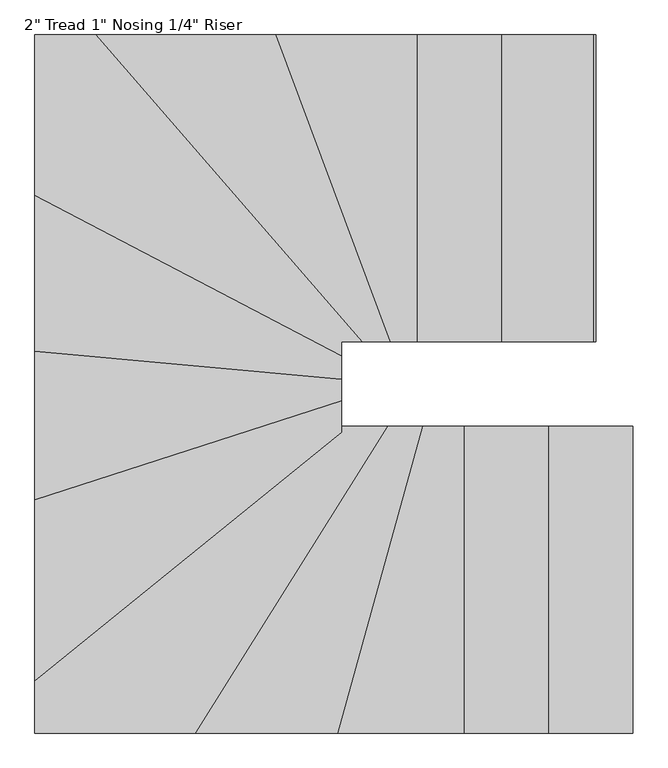
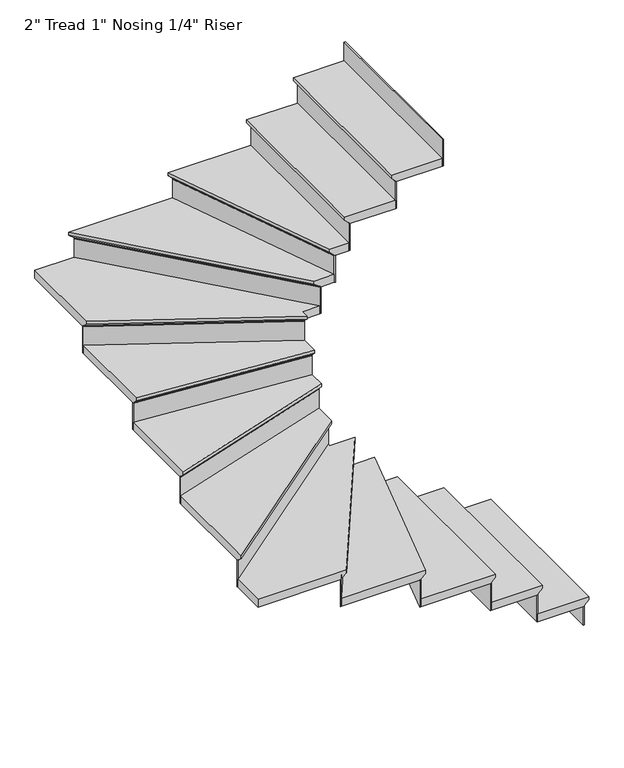
"""IFC4 building model written with IfcOpenShell, lengths in millimetres: stair flight geometry."""

from ifc_helpers import new_model, si_unit, origin, place, context, project, spatial, faceted_brep, source, transform, mapped, element, save


def stair_flight_22c751ce(model_context):
    return source(origin(), model_context, "Body", "Brep", [
        faceted_brep([(-7818.2848745, 5455.3549175, 319.6166667), (-7818.2848745, 5455.3549175, 338.6666667), (-7818.2848745, 4439.3549175, 338.6666667), (-7818.2848745, 4439.3549175, 319.6166667), (-7843.6848745, 5455.3549175, 294.2166667), (-7843.6848745, 4439.3549175, 294.2166667), (-8123.0848745, 5455.3549175, 338.6666667), (-8123.0848745, 4439.3549175, 338.6666667), (-7843.6848745, 4439.3549175, 287.8666667), (-8123.0848745, 4439.3549175, 287.8666667), (-8123.0848745, 5455.3549175, 287.8666667), (-7843.6848745, 5455.3549175, 287.8666667)], [[[0, 1, 2, 3]], [[4, 0, 3, 5]], [[2, 1, 6, 7]], [[8, 9, 10, 11]], [[2, 7, 9, 8, 5, 3]], [[8, 11, 4, 5]], [[6, 1, 0, 4, 11, 10]], [[7, 6, 10, 9]]]),
        faceted_brep([(-7843.6848745, 5455.3549175, 287.8666667), (-7843.6848745, 5455.3549175, 169.3333333), (-7850.0348745, 5455.3549175, 169.3333333), (-7850.0348745, 5455.3549175, 287.8666667), (-7843.6848745, 4439.3549175, 287.8666667), (-7850.0348745, 4439.3549175, 287.8666667), (-7850.0348745, 4439.3549175, 169.3333333), (-7843.6848745, 4439.3549175, 169.3333333)], [[[0, 1, 2, 3]], [[4, 5, 6, 7]], [[1, 0, 4, 7]], [[2, 1, 7, 6]], [[3, 2, 6, 5]], [[0, 3, 5, 4]]]),
        faceted_brep([(-8123.0848745, 5455.3549175, 457.2), (-8123.0848745, 5455.3549175, 287.8666667), (-8129.4348745, 5455.3549175, 287.8666667), (-8129.4348745, 5455.3549175, 457.2), (-8123.0848745, 4439.3549175, 457.2), (-8129.4348745, 4439.3549175, 457.2), (-8129.4348745, 4439.3549175, 287.8666667), (-8123.0848745, 4439.3549175, 287.8666667)], [[[0, 1, 2, 3]], [[4, 5, 6, 7]], [[1, 0, 4, 7]], [[2, 1, 7, 6]], [[3, 2, 6, 5]], [[0, 3, 5, 4]]]),
        faceted_brep([(-8097.6848745, 4439.3549175, 508.0), (-8097.6848745, 5455.3549175, 508.0), (-8402.4848745, 5455.3549175, 508.0), (-8402.4848745, 4439.3549175, 508.0), (-8123.0848745, 4439.3549175, 457.2), (-8402.4848745, 4439.3549175, 457.2), (-8402.4848745, 5455.3549175, 457.2), (-8123.0848745, 5455.3549175, 457.2), (-8123.0848745, 4439.3549175, 463.55), (-8097.6848745, 4439.3549175, 488.95), (-8123.0848745, 5455.3549175, 463.55), (-8097.6848745, 5455.3549175, 488.95)], [[[0, 1, 2, 3]], [[4, 5, 6, 7]], [[0, 3, 5, 4, 8, 9]], [[4, 7, 10, 8]], [[2, 1, 11, 10, 7, 6]], [[3, 2, 6, 5]], [[11, 1, 0, 9]], [[10, 11, 9, 8]]]),
        faceted_brep([(-8402.4848745, 5455.3549175, 626.5333333), (-8402.4848745, 5455.3549175, 457.2), (-8408.8348745, 5455.3549175, 457.2), (-8408.8348745, 5455.3549175, 626.5333333), (-8402.4848745, 4439.3549175, 626.5333333), (-8408.8348745, 4439.3549175, 626.5333333), (-8408.8348745, 4439.3549175, 457.2), (-8402.4848745, 4439.3549175, 457.2)], [[[0, 1, 2, 3]], [[4, 5, 6, 7]], [[1, 0, 4, 7]], [[2, 1, 7, 6]], [[3, 2, 6, 5]], [[0, 3, 5, 4]]]),
        faceted_brep([(-8377.0848745, 4439.3549175, 677.3333333), (-8377.0848745, 5455.3549175, 677.3333333), (-8542.1091668, 5455.3549175, 677.3333333), (-8823.5739204, 4439.3549175, 677.3333333), (-8402.4848745, 4439.3549175, 626.5333333), (-8823.5739204, 4439.3549175, 626.5333333), (-8542.1091668, 5455.3549175, 626.5333333), (-8402.4848745, 5455.3549175, 626.5333333), (-8402.4848745, 4439.3549175, 632.8833333), (-8377.0848745, 4439.3549175, 658.2833333), (-8402.4848745, 5455.3549175, 632.8833333), (-8377.0848745, 5455.3549175, 658.2833333)], [[[0, 1, 2, 3]], [[4, 5, 6, 7]], [[0, 3, 5, 4, 8, 9]], [[4, 7, 10, 8]], [[2, 1, 11, 10, 7, 6]], [[3, 2, 6, 5]], [[11, 1, 0, 9]], [[10, 11, 9, 8]]]),
        faceted_brep([(-8542.1091668, 5455.3549175, 795.8666667), (-8542.1091668, 5455.3549175, 626.5333333), (-8548.6983341, 5455.3549175, 626.5333333), (-8548.6983341, 5455.3549175, 795.8666667), (-8823.5739204, 4439.3549175, 795.8666667), (-8830.1630877, 4439.3549175, 795.8666667), (-8830.1630877, 4439.3549175, 626.5333333), (-8823.5739204, 4439.3549175, 626.5333333)], [[[0, 1, 2, 3]], [[4, 5, 6, 7]], [[1, 0, 4, 7]], [[2, 1, 7, 6]], [[3, 2, 6, 5]], [[0, 3, 5, 4]]]),
        faceted_brep([(-8797.2172513, 4439.3549175, 846.6666667), (-8515.7524978, 5455.3549175, 846.6666667), (-8660.9874718, 5455.3549175, 846.6666667), (-9297.7788575, 4439.3549175, 846.6666667), (-8823.5739204, 4439.3549175, 795.8666667), (-9297.7788575, 4439.3549175, 795.8666667), (-8660.9874718, 5455.3549175, 795.8666667), (-8542.1091668, 5455.3549175, 795.8666667), (-8823.5739204, 4439.3549175, 802.2166667), (-8797.2172513, 4439.3549175, 827.6166667), (-8542.1091668, 5455.3549175, 802.2166667), (-8515.7524978, 5455.3549175, 827.6166667)], [[[0, 1, 2, 3]], [[4, 5, 6, 7]], [[0, 3, 5, 4, 8, 9]], [[4, 7, 10, 8]], [[2, 1, 11, 10, 7, 6]], [[3, 2, 6, 5]], [[11, 1, 0, 9]], [[10, 11, 9, 8]]]),
        faceted_brep([(-8660.9874718, 5455.3549175, 965.2), (-8660.9874718, 5455.3549175, 795.8666667), (-8668.4816343, 5455.3549175, 795.8666667), (-8668.4816343, 5455.3549175, 965.2), (-9297.7788575, 4439.3549175, 965.2), (-9305.2730199, 4439.3549175, 965.2), (-9305.2730199, 4439.3549175, 795.8666667), (-9297.7788575, 4439.3549175, 795.8666667)], [[[0, 1, 2, 3]], [[4, 5, 6, 7]], [[1, 0, 4, 7]], [[2, 1, 7, 6]], [[3, 2, 6, 5]], [[0, 3, 5, 4]]]),
        faceted_brep([(-9799.482173, 4645.2534795, 1016.0), (-9799.482173, 4439.3549175, 1016.0), (-9267.8022075, 4439.3549175, 1016.0), (-8631.0108218, 5455.3549175, 1016.0), (-8783.482173, 5455.3549175, 1016.0), (-8783.482173, 5468.4858727, 1016.0), (-9799.482173, 4439.3549175, 965.2), (-9799.482173, 4645.2534795, 965.2), (-8783.482173, 5468.4858727, 965.2), (-8783.482173, 5455.3549175, 965.2), (-8660.9874718, 5455.3549175, 965.2), (-9297.7788575, 4439.3549175, 965.2), (-8660.9874718, 5455.3549175, 971.55), (-9297.7788575, 4439.3549175, 971.55), (-8631.0108218, 5455.3549175, 996.95), (-9267.8022075, 4439.3549175, 996.95)], [[[0, 1, 2, 3, 4, 5]], [[6, 7, 8, 9, 10, 11]], [[1, 0, 7, 6]], [[11, 10, 12, 13]], [[4, 3, 14, 12, 10, 9]], [[0, 5, 8, 7]], [[14, 3, 2, 15]], [[12, 14, 15, 13]], [[2, 1, 6, 11, 13, 15]], [[5, 4, 9, 8]]]),
        faceted_brep([(-8783.482173, 5468.4858727, 1134.5333333), (-8783.482173, 5468.4858727, 965.2), (-8783.482173, 5476.6587307, 965.2), (-8783.482173, 5476.6587307, 1134.5333333), (-9799.482173, 4645.2534795, 1134.5333333), (-9799.482173, 4653.4263375, 1134.5333333), (-9799.482173, 4653.4263375, 965.2), (-9799.482173, 4645.2534795, 965.2)], [[[0, 1, 2, 3]], [[4, 5, 6, 7]], [[1, 0, 4, 7]], [[2, 1, 7, 6]], [[3, 2, 6, 5]], [[0, 3, 5, 4]]]),
        faceted_brep([(-9799.482173, 4612.5620474, 1185.3333333), (-8783.482173, 5435.7944406, 1185.3333333), (-8783.482173, 5565.6796441, 1185.3333333), (-9799.482173, 5238.9822106, 1185.3333333), (-9799.482173, 4645.2534795, 1134.5333333), (-9799.482173, 5238.9822106, 1134.5333333), (-8783.482173, 5565.6796441, 1134.5333333), (-8783.482173, 5468.4858727, 1134.5333333), (-9799.482173, 4645.2534795, 1140.8833333), (-9799.482173, 4612.5620474, 1166.2833333), (-8783.482173, 5468.4858727, 1140.8833333), (-8783.482173, 5435.7944406, 1166.2833333)], [[[0, 1, 2, 3]], [[4, 5, 6, 7]], [[0, 3, 5, 4, 8, 9]], [[4, 7, 10, 8]], [[3, 2, 6, 5]], [[11, 1, 0, 9]], [[10, 11, 9, 8]], [[2, 1, 11, 10, 7, 6]]]),
        faceted_brep([(-8783.482173, 5565.6796441, 1303.8666667), (-8783.482173, 5565.6796441, 1134.5333333), (-8783.482173, 5572.3498531, 1134.5333333), (-8783.482173, 5572.3498531, 1303.8666667), (-9799.482173, 5238.9822106, 1303.8666667), (-9799.482173, 5245.6524196, 1303.8666667), (-9799.482173, 5245.6524196, 1134.5333333), (-9799.482173, 5238.9822106, 1134.5333333)], [[[0, 1, 2, 3]], [[4, 5, 6, 7]], [[1, 0, 4, 7]], [[2, 1, 7, 6]], [[3, 2, 6, 5]], [[0, 3, 5, 4]]]),
        faceted_brep([(-9799.482173, 5212.3013746, 1354.6666667), (-8783.482173, 5538.9988082, 1354.6666667), (-8783.482173, 5636.5023377, 1354.6666667), (-9799.482173, 5728.3284264, 1354.6666667), (-9799.482173, 5238.9822106, 1303.8666667), (-9799.482173, 5728.3284264, 1303.8666667), (-8783.482173, 5636.5023377, 1303.8666667), (-8783.482173, 5565.6796441, 1303.8666667), (-9799.482173, 5238.9822106, 1310.2166667), (-9799.482173, 5212.3013746, 1335.6166667), (-8783.482173, 5565.6796441, 1310.2166667), (-8783.482173, 5538.9988082, 1335.6166667)], [[[0, 1, 2, 3]], [[4, 5, 6, 7]], [[0, 3, 5, 4, 8, 9]], [[4, 7, 10, 8]], [[2, 1, 11, 10, 7, 6]], [[3, 2, 6, 5]], [[11, 1, 0, 9]], [[10, 11, 9, 8]]]),
        faceted_brep([(-8783.482173, 5636.5023377, 1473.2), (-8783.482173, 5636.5023377, 1303.8666667), (-8783.482173, 5642.8782201, 1303.8666667), (-8783.482173, 5642.8782201, 1473.2), (-9799.482173, 5728.3284264, 1473.2), (-9799.482173, 5734.7043088, 1473.2), (-9799.482173, 5734.7043088, 1303.8666667), (-9799.482173, 5728.3284264, 1303.8666667)], [[[0, 1, 2, 3]], [[4, 5, 6, 7]], [[1, 0, 4, 7]], [[2, 1, 7, 6]], [[3, 2, 6, 5]], [[0, 3, 5, 4]]]),
        faceted_brep([(-9799.482173, 5702.8248969, 1524.0), (-8783.482173, 5610.9988082, 1524.0), (-8783.482173, 5717.0988353, 1524.0), (-9799.482173, 6249.3577674, 1524.0), (-9799.482173, 5728.3284264, 1473.2), (-9799.482173, 6249.3577674, 1473.2), (-8783.482173, 5717.0988353, 1473.2), (-8783.482173, 5636.5023377, 1473.2), (-9799.482173, 5728.3284264, 1479.55), (-9799.482173, 5702.8248969, 1504.95), (-8783.482173, 5636.5023377, 1479.55), (-8783.482173, 5610.9988082, 1504.95)], [[[0, 1, 2, 3]], [[4, 5, 6, 7]], [[0, 3, 5, 4, 8, 9]], [[4, 7, 10, 8]], [[3, 2, 6, 5]], [[11, 1, 0, 9]], [[10, 11, 9, 8]], [[2, 1, 11, 10, 7, 6]]]),
        faceted_brep([(-8783.482173, 5717.0988353, 1642.5333333), (-8783.482173, 5717.0988353, 1473.2), (-8783.482173, 5724.2674398, 1473.2), (-8783.482173, 5724.2674398, 1642.5333333), (-9799.482173, 6249.3577674, 1642.5333333), (-9799.482173, 6256.5263718, 1642.5333333), (-9799.482173, 6256.5263718, 1473.2), (-9799.482173, 6249.3577674, 1473.2)], [[[0, 1, 2, 3]], [[4, 5, 6, 7]], [[1, 0, 4, 7]], [[2, 1, 7, 6]], [[3, 2, 6, 5]], [[0, 3, 5, 4]]]),
        faceted_brep([(-9562.9934983, 6750.7549175, 1693.3333333), (-9799.482173, 6750.7549175, 1693.3333333), (-9799.482173, 6220.6833497, 1693.3333333), (-8783.482173, 5688.4244176, 1693.3333333), (-8783.482173, 5734.7549175, 1693.3333333), (-8680.4598937, 5734.7549175, 1693.3333333), (-9799.482173, 6750.7549175, 1642.5333333), (-9562.9934983, 6750.7549175, 1642.5333333), (-8680.4598937, 5734.7549175, 1642.5333333), (-8783.482173, 5734.7549175, 1642.5333333), (-8783.482173, 5717.0988353, 1642.5333333), (-9799.482173, 6249.3577674, 1642.5333333), (-8783.482173, 5717.0988353, 1648.8833333), (-9799.482173, 6249.3577674, 1648.8833333), (-8783.482173, 5688.4244176, 1674.2833333), (-9799.482173, 6220.6833497, 1674.2833333)], [[[0, 1, 2, 3, 4, 5]], [[6, 7, 8, 9, 10, 11]], [[1, 0, 7, 6]], [[11, 10, 12, 13]], [[4, 3, 14, 12, 10, 9]], [[0, 5, 8, 7]], [[14, 3, 2, 15]], [[12, 14, 15, 13]], [[2, 1, 6, 11, 13, 15]], [[5, 4, 9, 8]]]),
        faceted_brep([(-8680.4598937, 5734.7549175, 1811.8666667), (-8680.4598937, 5734.7549175, 1642.5333333), (-8672.0487739, 5734.7549175, 1642.5333333), (-8672.0487739, 5734.7549175, 1811.8666667), (-9562.9934983, 6750.7549175, 1811.8666667), (-9554.5823785, 6750.7549175, 1811.8666667), (-9554.5823785, 6750.7549175, 1642.5333333), (-9562.9934983, 6750.7549175, 1642.5333333)], [[[0, 1, 2, 3]], [[4, 5, 6, 7]], [[1, 0, 4, 7]], [[2, 1, 7, 6]], [[3, 2, 6, 5]], [[0, 3, 5, 4]]]),
        faceted_brep([(-9596.6379775, 6750.7549175, 1862.6666667), (-8714.1043729, 5734.7549175, 1862.6666667), (-8594.868364, 5734.7549175, 1862.6666667), (-8974.0365508, 6750.7549175, 1862.6666667), (-9562.9934983, 6750.7549175, 1811.8666667), (-8974.0365508, 6750.7549175, 1811.8666667), (-8594.868364, 5734.7549175, 1811.8666667), (-8680.4598937, 5734.7549175, 1811.8666667), (-9562.9934983, 6750.7549175, 1818.2166667), (-9596.6379775, 6750.7549175, 1843.6166667), (-8680.4598937, 5734.7549175, 1818.2166667), (-8714.1043729, 5734.7549175, 1843.6166667)], [[[0, 1, 2, 3]], [[4, 5, 6, 7]], [[0, 3, 5, 4, 8, 9]], [[4, 7, 10, 8]], [[2, 1, 11, 10, 7, 6]], [[3, 2, 6, 5]], [[11, 1, 0, 9]], [[10, 11, 9, 8]]]),
        faceted_brep([(-8594.868364, 5734.7549175, 1981.2), (-8594.868364, 5734.7549175, 1811.8666667), (-8588.0905725, 5734.7549175, 1811.8666667), (-8588.0905725, 5734.7549175, 1981.2), (-8974.0365508, 6750.7549175, 1981.2), (-8967.2587593, 6750.7549175, 1981.2), (-8967.2587593, 6750.7549175, 1811.8666667), (-8974.0365508, 6750.7549175, 1811.8666667)], [[[0, 1, 2, 3]], [[4, 5, 6, 7]], [[1, 0, 4, 7]], [[2, 1, 7, 6]], [[3, 2, 6, 5]], [[0, 3, 5, 4]]]),
        faceted_brep([(-9001.1477168, 6750.7549175, 2032.0), (-8621.9795299, 5734.7549175, 2032.0), (-8506.4806206, 5734.7549175, 2032.0), (-8506.4806206, 6750.7549175, 2032.0), (-8974.0365508, 6750.7549175, 1981.2), (-8506.4806206, 6750.7549175, 1981.2), (-8506.4806206, 5734.7549175, 1981.2), (-8594.868364, 5734.7549175, 1981.2), (-8974.0365508, 6750.7549175, 1987.55), (-9001.1477168, 6750.7549175, 2012.95), (-8594.868364, 5734.7549175, 1987.55), (-8621.9795299, 5734.7549175, 2012.95)], [[[0, 1, 2, 3]], [[4, 5, 6, 7]], [[0, 3, 5, 4, 8, 9]], [[4, 7, 10, 8]], [[2, 1, 11, 10, 7, 6]], [[3, 2, 6, 5]], [[11, 1, 0, 9]], [[10, 11, 9, 8]]]),
        faceted_brep([(-8506.4806206, 5734.7549175, 2150.5333333), (-8506.4806206, 5734.7549175, 1981.2), (-8500.1306206, 5734.7549175, 1981.2), (-8500.1306206, 5734.7549175, 2150.5333333), (-8506.4806206, 6750.7549175, 2150.5333333), (-8500.1306206, 6750.7549175, 2150.5333333), (-8500.1306206, 6750.7549175, 1981.2), (-8506.4806206, 6750.7549175, 1981.2)], [[[0, 1, 2, 3]], [[4, 5, 6, 7]], [[1, 0, 4, 7]], [[2, 1, 7, 6]], [[3, 2, 6, 5]], [[0, 3, 5, 4]]]),
        faceted_brep([(-8531.8806206, 6750.7549175, 2201.3333333), (-8531.8806206, 5734.7549175, 2201.3333333), (-8227.0806206, 5734.7549175, 2201.3333333), (-8227.0806206, 6750.7549175, 2201.3333333), (-8506.4806206, 6750.7549175, 2150.5333333), (-8227.0806206, 6750.7549175, 2150.5333333), (-8227.0806206, 5734.7549175, 2150.5333333), (-8506.4806206, 5734.7549175, 2150.5333333), (-8506.4806206, 6750.7549175, 2156.8833333), (-8531.8806206, 6750.7549175, 2182.2833333), (-8506.4806206, 5734.7549175, 2156.8833333), (-8531.8806206, 5734.7549175, 2182.2833333)], [[[0, 1, 2, 3]], [[4, 5, 6, 7]], [[0, 3, 5, 4, 8, 9]], [[4, 7, 10, 8]], [[2, 1, 11, 10, 7, 6]], [[3, 2, 6, 5]], [[11, 1, 0, 9]], [[10, 11, 9, 8]]]),
        faceted_brep([(-8227.0806206, 5734.7549175, 2319.8666667), (-8227.0806206, 5734.7549175, 2150.5333333), (-8220.7306206, 5734.7549175, 2150.5333333), (-8220.7306206, 5734.7549175, 2319.8666667), (-8227.0806206, 6750.7549175, 2319.8666667), (-8220.7306206, 6750.7549175, 2319.8666667), (-8220.7306206, 6750.7549175, 2150.5333333), (-8227.0806206, 6750.7549175, 2150.5333333)], [[[0, 1, 2, 3]], [[4, 5, 6, 7]], [[1, 0, 4, 7]], [[2, 1, 7, 6]], [[3, 2, 6, 5]], [[0, 3, 5, 4]]]),
        faceted_brep([(-7947.6806206, 5734.7549175, 2489.2), (-7947.6806206, 5734.7549175, 2319.8666667), (-7941.3306206, 5734.7549175, 2319.8666667), (-7941.3306206, 5734.7549175, 2489.2), (-7947.6806206, 6750.7549175, 2489.2), (-7941.3306206, 6750.7549175, 2489.2), (-7941.3306206, 6750.7549175, 2319.8666667), (-7947.6806206, 6750.7549175, 2319.8666667)], [[[0, 1, 2, 3]], [[4, 5, 6, 7]], [[1, 0, 4, 7]], [[2, 1, 7, 6]], [[3, 2, 6, 5]], [[0, 3, 5, 4]]]),
        faceted_brep([(-8252.4806206, 6750.7549175, 2370.6666667), (-8252.4806206, 5734.7549175, 2370.6666667), (-7947.6806206, 5734.7549175, 2370.6666667), (-7947.6806206, 6750.7549175, 2370.6666667), (-8227.0806206, 6750.7549175, 2319.8666667), (-7947.6806206, 6750.7549175, 2319.8666667), (-7947.6806206, 5734.7549175, 2319.8666667), (-8227.0806206, 5734.7549175, 2319.8666667), (-8227.0806206, 6750.7549175, 2326.2166667), (-8252.4806206, 6750.7549175, 2351.6166667), (-8227.0806206, 5734.7549175, 2326.2166667), (-8252.4806206, 5734.7549175, 2351.6166667)], [[[0, 1, 2, 3]], [[4, 5, 6, 7]], [[0, 3, 5, 4, 8, 9]], [[4, 7, 10, 8]], [[2, 1, 11, 10, 7, 6]], [[3, 2, 6, 5]], [[11, 1, 0, 9]], [[10, 11, 9, 8]]]),
    ])


if __name__ == "__main__":
    model = new_model("IFC4")
    model_context = context("Model", 3, world=origin())
    ifc_project = project(units=[si_unit("LENGTHUNIT", "METRE", prefix="MILLI")], contexts=[model_context])
    site = spatial("IfcSite", under=ifc_project)
    building = spatial("IfcBuilding", under=site)
    placement = place(None, origin())
    stair_flight_shape = stair_flight_22c751ce(model_context)
    element("IfcStairFlight", 1, ObjectType="2\" Tread 1\" Nosing 1/4\" Riser", at=placement, inside=building, context=model_context, shape_type="MappedRepresentation", body=[
        mapped(stair_flight_shape, transform((0.0, 0.0, 0.0), x_axis=(1.0, 0.0, 0.0), y_axis=(0.0, 1.0, 0.0), z_axis=(0.0, 0.0, 1.0))),
    ])
    save(model, "model.ifc")
